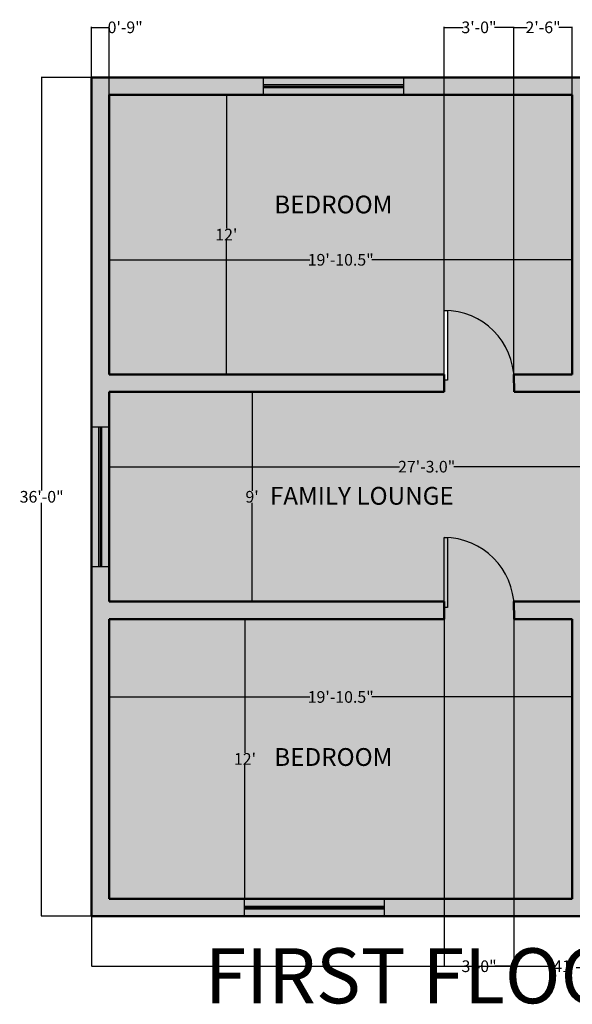
# Model space of a CAD drawing. Units: inches. Extents: x 1379 to 6665, y -118 to 1026.
# Tile 27 of 29: x 6130 to 6415, y 26 to 533. Entities that reach past the tile are written whole.
import ezdxf

# ---------------------------------------------------------------- set-up
doc = ezdxf.new("R2010")
doc.units = ezdxf.units.IN
doc.header["$MEASUREMENT"] = 0
for name, color, linetype, lineweight in [('A-ANNO-DIMS', 2, 'Continuous', 18), ('A-ANNO-TEXT', 7, 'Continuous', 35), ('A-AREA-IDEN', 7, 'Continuous', 25), ('A-DOOR', 1, 'Continuous', 25), ('A-FLOR-PATT', 252, 'Continuous', 13), ('A-GLAZ', 2, 'Continuous', 25), ('A-WALL', 7, 'Continuous', 50), ('A-WALL-PATT', 8, 'Continuous', 13)]:
    doc.layers.add(name, color=color, linetype=linetype, lineweight=lineweight)
doc.styles.get("Standard").update_dxf_attribs({"font": 'arial.ttf'})
doc.dimstyles.get("Standard").update_dxf_attribs({"dimtxt": 6, "dimasz": 0.18, "dimexe": 0.18, "dimexo": 0.0625, "dimgap": 0.09, "dimtad": 0, "dimtih": 1, "dimtoh": 1, "dimdec": 1, "dimzin": 0, "dimdsep": 46, "dimlunit": 3, "dimtxsty": 'Standard', "dimcen": 0.09, "dimclrt": 250, "dimadec": 0, "dimazin": 0, "dimtfac": 1, "dimtdec": 1, "dimtofl": 0, "dimtmove": 0, "dimatfit": 3, "dimfxl": 1, "dimtolj": 1, "dimtzin": 0, "dimarcsym": 0})

# ---------------------------------------------------------------- blocks, each defined once
blk = doc.blocks.new('*U3')
for p, q in [((0, 0), (0, -6)), ((36, 0), (36, -6))]:
    blk.add_line(p, q)
blk.add_lwpolyline([(0, 0), (0, 36), (1.75, 36), (1.75, 0)], close=True)
blk.add_arc((0, 0), 36, 0, 90)
blk = doc.blocks.new('*D76')
at = {"layer": 'A-ANNO-DIMS', "color": 0, "lineweight": -2, "transparency": 16777216}
for p, q in [((6235.37, 494.64), (6236.93, 494.64)), ((6236.75, 494.46), (6236.75, 425.74)), ((6236.75, 350.82), (6236.75, 419.54)), ((6235.37, 350.64), (6236.93, 350.64))]:
    blk.add_line(p, q, dxfattribs=at)
at = {"layer": 'A-ANNO-DIMS', "color": 0, "transparency": 16777216}
for points in [[(6236.72, 494.46), (6236.78, 494.46), (6236.75, 494.64)], [(6236.72, 350.82), (6236.78, 350.82), (6236.75, 350.64)]]:
    blk.add_solid(points, dxfattribs=at)
at = {"layer": 'Defpoints', "color": 0, "transparency": 16777216}
for p in [(6235.31, 494.64), (6235.31, 350.64), (6236.75, 350.64)]:
    blk.add_point(p, dxfattribs=at)
at = {"layer": 'A-ANNO-DIMS', "color": 0, "transparency": 16777216, "insert": (6236.75, 422.64), "char_height": 6, "attachment_point": 5}
blk.add_mtext("\\A1;12'", dxfattribs=at)
blk = doc.blocks.new('*D77')
at = {"layer": 'A-ANNO-DIMS', "color": 0, "lineweight": -2, "transparency": 16777216}
for p, q in [((6176.4, 417.36), (6176.4, 409.5)), ((6414.9, 417.36), (6414.9, 409.5)), ((6176.58, 409.68), (6279.71, 409.68)), ((6414.72, 409.68), (6311.59, 409.68))]:
    blk.add_line(p, q, dxfattribs=at)
at = {"layer": 'A-ANNO-DIMS', "color": 0, "transparency": 16777216}
for points in [[(6176.58, 409.71), (6176.58, 409.65), (6176.4, 409.68)], [(6414.72, 409.71), (6414.72, 409.65), (6414.9, 409.68)]]:
    blk.add_solid(points, dxfattribs=at)
at = {"layer": 'Defpoints', "color": 0, "transparency": 16777216}
for p in [(6176.4, 417.42), (6414.9, 417.42), (6414.9, 409.68)]:
    blk.add_point(p, dxfattribs=at)
at = {"layer": 'A-ANNO-DIMS', "color": 0, "transparency": 16777216, "insert": (6295.65, 409.68), "char_height": 6, "attachment_point": 5}
blk.add_mtext('\\A1;19\'-10.5"', dxfattribs=at)
blk = doc.blocks.new('*D78')
at = {"layer": 'A-ANNO-DIMS', "color": 0, "lineweight": -2, "transparency": 16777216}
for p, q in [((6281.87, 341.64), (6249.82, 341.64)), ((6250, 341.46), (6250, 290.79)), ((6250, 233.82), (6250, 284.49)), ((6281.87, 233.64), (6249.82, 233.64))]:
    blk.add_line(p, q, dxfattribs=at)
at = {"layer": 'A-ANNO-DIMS', "color": 0, "transparency": 16777216}
for points in [[(6249.97, 341.46), (6250.03, 341.46), (6250, 341.64)], [(6249.97, 233.82), (6250.03, 233.82), (6250, 233.64)]]:
    blk.add_solid(points, dxfattribs=at)
at = {"layer": 'Defpoints', "color": 0, "transparency": 16777216}
for p in [(6281.94, 341.64), (6250, 233.64), (6281.94, 233.64)]:
    blk.add_point(p, dxfattribs=at)
at = {"layer": 'A-ANNO-DIMS', "color": 0, "transparency": 16777216, "insert": (6250, 287.64), "char_height": 6, "attachment_point": 5}
blk.add_mtext("\\A1;9'", dxfattribs=at)
blk = doc.blocks.new('*D80')
at = {"layer": 'A-ANNO-DIMS', "color": 0, "lineweight": -2, "transparency": 16777216}
for p, q in [((6176.4, 282.22), (6176.4, 303.33)), ((6176.58, 303.15), (6325.96, 303.15)), ((6503.22, 303.15), (6353.84, 303.15)), ((6503.4, 282.22), (6503.4, 303.33))]:
    blk.add_line(p, q, dxfattribs=at)
at = {"layer": 'A-ANNO-DIMS', "color": 0, "transparency": 16777216}
for points in [[(6176.58, 303.18), (6176.58, 303.12), (6176.4, 303.15)], [(6503.22, 303.18), (6503.22, 303.12), (6503.4, 303.15)]]:
    blk.add_solid(points, dxfattribs=at)
at = {"layer": 'Defpoints', "color": 0, "transparency": 16777216}
for p in [(6503.4, 303.15), (6176.4, 282.16), (6503.4, 282.16)]:
    blk.add_point(p, dxfattribs=at)
at = {"layer": 'A-ANNO-DIMS', "color": 0, "transparency": 16777216, "insert": (6339.9, 303.15), "char_height": 6, "attachment_point": 5}
blk.add_mtext('\\A1;27\'-3.0"', dxfattribs=at)
blk = doc.blocks.new('*D87')
at = {"layer": 'A-ANNO-DIMS', "color": 0, "lineweight": -2, "transparency": 16777216}
for p, q in [((6262.59, 224.64), (6246.17, 224.64)), ((6246.35, 224.46), (6246.35, 155.74)), ((6246.35, 80.82), (6246.35, 149.54)), ((6262.59, 80.64), (6246.17, 80.64))]:
    blk.add_line(p, q, dxfattribs=at)
at = {"layer": 'A-ANNO-DIMS', "color": 0, "transparency": 16777216}
for points in [[(6246.32, 224.46), (6246.38, 224.46), (6246.35, 224.64)], [(6246.32, 80.82), (6246.38, 80.82), (6246.35, 80.64)]]:
    blk.add_solid(points, dxfattribs=at)
at = {"layer": 'Defpoints', "color": 0, "transparency": 16777216}
for p in [(6262.65, 224.64), (6246.35, 80.64), (6262.65, 80.64)]:
    blk.add_point(p, dxfattribs=at)
at = {"layer": 'A-ANNO-DIMS', "color": 0, "transparency": 16777216, "insert": (6246.35, 152.64), "char_height": 6, "attachment_point": 5}
blk.add_mtext("\\A1;12'", dxfattribs=at)
blk = doc.blocks.new('*D88')
at = {"layer": 'A-ANNO-DIMS', "color": 0, "lineweight": -2, "transparency": 16777216}
for p, q in [((6176.4, 163.43), (6176.4, 184.73)), ((6176.58, 184.55), (6279.71, 184.55)), ((6414.72, 184.55), (6311.59, 184.55)), ((6414.9, 164.7), (6414.9, 184.73))]:
    blk.add_line(p, q, dxfattribs=at)
at = {"layer": 'A-ANNO-DIMS', "color": 0, "transparency": 16777216}
for points in [[(6176.58, 184.58), (6176.58, 184.52), (6176.4, 184.55)], [(6414.72, 184.58), (6414.72, 184.52), (6414.9, 184.55)]]:
    blk.add_solid(points, dxfattribs=at)
at = {"layer": 'Defpoints', "color": 0, "transparency": 16777216}
for p in [(6414.9, 184.55), (6176.4, 163.37), (6414.9, 164.64)]:
    blk.add_point(p, dxfattribs=at)
at = {"layer": 'A-ANNO-DIMS', "color": 0, "transparency": 16777216, "insert": (6295.65, 184.55), "char_height": 6, "attachment_point": 5}
blk.add_mtext('\\A1;19\'-10.5"', dxfattribs=at)
blk = doc.blocks.new('WIN-1800')
for p, q in [((0, 0.73), (72, 0.73)), ((0, 0), (72, 0))]:
    blk.add_line(p, q)
blk = doc.blocks.new('*D136')
at = {"layer": 'A-ANNO-DIMS', "color": 0, "lineweight": -2, "transparency": 16777216}
for p, q in [((6167.4, 71.58), (6167.4, 45.71)), ((6665.4, 71.58), (6665.4, 45.71)), ((6167.58, 45.89), (6405.89, 45.89)), ((6665.22, 45.89), (6426.92, 45.89))]:
    blk.add_line(p, q, dxfattribs=at)
at = {"layer": 'A-ANNO-DIMS', "color": 0, "transparency": 16777216}
for points in [[(6167.58, 45.92), (6167.58, 45.86), (6167.4, 45.89)], [(6665.22, 45.92), (6665.22, 45.86), (6665.4, 45.89)]]:
    blk.add_solid(points, dxfattribs=at)
at = {"layer": 'Defpoints', "color": 0, "transparency": 16777216}
for p in [(6167.4, 71.64), (6665.4, 71.64), (6665.4, 45.89)]:
    blk.add_point(p, dxfattribs=at)
at = {"layer": 'A-ANNO-DIMS', "color": 250, "transparency": 16777216, "insert": (6416.4, 45.89), "char_height": 6, "attachment_point": 5}
blk.add_mtext('\\A1;41\'-6"', dxfattribs=at)
blk = doc.blocks.new('*D137')
at = {"layer": 'A-ANNO-DIMS', "color": 0, "lineweight": -2, "transparency": 16777216}
for p, q in [((6167.34, 503.64), (6141.47, 503.64)), ((6141.65, 503.46), (6141.65, 290.8)), ((6141.65, 71.82), (6141.65, 284.48)), ((6167.34, 71.64), (6141.47, 71.64))]:
    blk.add_line(p, q, dxfattribs=at)
at = {"layer": 'A-ANNO-DIMS', "color": 0, "transparency": 16777216}
for points in [[(6141.62, 503.46), (6141.68, 503.46), (6141.65, 503.64)], [(6141.62, 71.82), (6141.68, 71.82), (6141.65, 71.64)]]:
    blk.add_solid(points, dxfattribs=at)
at = {"layer": 'Defpoints', "color": 0, "transparency": 16777216}
for p in [(6141.65, 503.64), (6167.4, 503.64), (6167.4, 71.64)]:
    blk.add_point(p, dxfattribs=at)
at = {"layer": 'A-ANNO-DIMS', "color": 250, "transparency": 16777216, "insert": (6141.65, 287.64), "char_height": 6, "attachment_point": 5}
blk.add_mtext('\\A1;36\'-0"', dxfattribs=at)
blk = doc.blocks.new('*D138')
at = {"layer": 'A-ANNO-DIMS', "color": 0, "lineweight": -2, "transparency": 16777216}
for p, q in [((6167.4, 503.7), (6167.4, 529.57)), ((6167.58, 529.39), (6176.22, 529.39)), ((6176.4, 494.7), (6176.4, 529.57)), ((6176.4, 529.39), (6176.58, 529.39))]:
    blk.add_line(p, q, dxfattribs=at)
at = {"layer": 'A-ANNO-DIMS', "color": 0, "transparency": 16777216}
for points in [[(6167.58, 529.42), (6167.58, 529.36), (6167.4, 529.39)], [(6176.22, 529.42), (6176.22, 529.36), (6176.4, 529.39)]]:
    blk.add_solid(points, dxfattribs=at)
at = {"layer": 'Defpoints', "color": 0, "transparency": 16777216}
for p in [(6176.4, 529.39), (6167.4, 503.64), (6176.4, 494.64)]:
    blk.add_point(p, dxfattribs=at)
at = {"layer": 'A-ANNO-DIMS', "color": 250, "transparency": 16777216, "insert": (6184.65, 529.39), "char_height": 6, "attachment_point": 5}
blk.add_mtext('\\A1;0\'-9"', dxfattribs=at)
blk = doc.blocks.new('*D143')
at = {"layer": 'A-ANNO-DIMS', "color": 0, "lineweight": -2, "transparency": 16777216}
for p, q in [((6384.78, 350.7), (6384.78, 529.57)), ((6384.96, 529.39), (6391.72, 529.39)), ((6414.72, 529.39), (6407.96, 529.39)), ((6414.9, 350.7), (6414.9, 529.57))]:
    blk.add_line(p, q, dxfattribs=at)
at = {"layer": 'A-ANNO-DIMS', "color": 0, "transparency": 16777216}
for points in [[(6384.96, 529.42), (6384.96, 529.36), (6384.78, 529.39)], [(6414.72, 529.42), (6414.72, 529.36), (6414.9, 529.39)]]:
    blk.add_solid(points, dxfattribs=at)
at = {"layer": 'Defpoints', "color": 0, "transparency": 16777216}
for p in [(6414.9, 529.39), (6384.78, 350.64), (6414.9, 350.64)]:
    blk.add_point(p, dxfattribs=at)
at = {"layer": 'A-ANNO-DIMS', "color": 250, "transparency": 16777216, "insert": (6399.84, 529.39), "char_height": 6, "attachment_point": 5}
blk.add_mtext('\\A1;2\'-6"', dxfattribs=at)
blk = doc.blocks.new('*D144')
at = {"layer": 'A-ANNO-DIMS', "color": 0, "lineweight": -2, "transparency": 16777216}
for p, q in [((6348.9, 350.7), (6348.9, 529.57)), ((6349.08, 529.39), (6358.78, 529.39)), ((6384.6, 529.39), (6374.9, 529.39)), ((6384.78, 350.7), (6384.78, 529.57))]:
    blk.add_line(p, q, dxfattribs=at)
at = {"layer": 'A-ANNO-DIMS', "color": 0, "transparency": 16777216}
for points in [[(6349.08, 529.42), (6349.08, 529.36), (6348.9, 529.39)], [(6384.6, 529.42), (6384.6, 529.36), (6384.78, 529.39)]]:
    blk.add_solid(points, dxfattribs=at)
at = {"layer": 'Defpoints', "color": 0, "transparency": 16777216}
for p in [(6384.78, 529.39), (6348.9, 350.64), (6384.78, 350.64)]:
    blk.add_point(p, dxfattribs=at)
at = {"layer": 'A-ANNO-DIMS', "color": 250, "transparency": 16777216, "insert": (6366.84, 529.39), "char_height": 6, "attachment_point": 5}
blk.add_mtext('\\A1;3\'-0"', dxfattribs=at)
blk = doc.blocks.new('*D145')
at = {"layer": 'A-ANNO-DIMS', "color": 0, "lineweight": -2, "transparency": 16777216}
for p, q in [((6348.9, 233.58), (6348.9, 45.71)), ((6384.87, 233.58), (6384.87, 45.71)), ((6349.08, 45.89), (6358.82, 45.89)), ((6384.69, 45.89), (6374.95, 45.89))]:
    blk.add_line(p, q, dxfattribs=at)
at = {"layer": 'A-ANNO-DIMS', "color": 0, "transparency": 16777216}
for points in [[(6349.08, 45.92), (6349.08, 45.86), (6348.9, 45.89)], [(6384.69, 45.92), (6384.69, 45.86), (6384.87, 45.89)]]:
    blk.add_solid(points, dxfattribs=at)
at = {"layer": 'Defpoints', "color": 0, "transparency": 16777216}
for p in [(6348.9, 233.64), (6384.87, 233.64), (6384.87, 45.89)]:
    blk.add_point(p, dxfattribs=at)
at = {"layer": 'A-ANNO-DIMS', "color": 250, "transparency": 16777216, "insert": (6366.89, 45.89), "char_height": 6, "attachment_point": 5}
blk.add_mtext('\\A1;3\'-0"', dxfattribs=at)

msp = doc.modelspace()

# ---------------------------------------------------------------- hatches: boundary and pattern name
at = {"layer": 'A-FLOR-PATT', "transparency": 33554590}
h = msp.add_hatch(color=256, dxfattribs=at)
h.dxf.hatch_style = 1
h.paths.add_polyline_path([(6176.4, 382.14), (6176.4, 494.64), (6255.9, 494.64), (6255.9, 503.64), (6167.4, 503.64), (6167.4, 391.14), (6167.4, 323.64), (6176.4, 323.64), (6176.4, 341.64), (6348.9, 341.64), (6348.9, 350.64), (6176.4, 350.64)])
h.paths.add_polyline_path([(6348.9, 233.64), (6176.4, 233.64), (6176.4, 251.64), (6167.4, 251.64), (6167.4, 71.64), (6246.02, 71.64), (6246.02, 80.64), (6176.4, 80.64), (6176.4, 224.64), (6348.9, 224.64)])
h.paths.add_polyline_path([(6443.4, 80.64), (6419.4, 80.64), (6419.4, 164.64), (6467.4, 164.64), (6467.4, 169.14), (6419.4, 169.14), (6419.4, 224.64), (6419.4, 233.64), (6384.87, 233.64), (6384.9, 224.64), (6414.9, 224.64), (6414.9, 80.64), (6318.02, 80.64), (6318.02, 71.64), (6443.4, 71.64)])
h.paths.add_polyline_path([(6552.9, 80.64), (6500.4, 80.64), (6500.4, 169.14), (6491.4, 169.14), (6491.4, 164.64), (6491.4, 80.64), (6467.4, 80.64), (6467.4, 71.64), (6503.4, 71.64), (6552.9, 71.64)])
h.paths.add_polyline_path([(6665.4, 188.64), (6656.4, 188.64), (6656.4, 176.64), (6626.4, 176.64), (6626.4, 172.14), (6656.4, 172.14), (6656.4, 80.64), (6624.9, 80.64), (6624.9, 71.64), (6665.4, 71.64)])
h.paths.add_polyline_path([(6665.4, 503.64), (6614.4, 503.64), (6614.4, 494.64), (6656.4, 494.64), (6656.4, 374.64), (6608.4, 374.64), (6608.4, 370.14), (6656.4, 370.14), (6656.4, 331.14), (6512.4, 331.14), (6503.4, 331.14), (6503.4, 322.14), (6503.4, 317.64), (6656.4, 317.64), (6656.4, 233.64), (6503.4, 233.64), (6455.4, 233.64), (6455.4, 224.64), (6503.4, 224.64), (6567.9, 224.64), (6567.9, 176.64), (6540.4, 176.64), (6540.4, 172.14), (6567.9, 172.14), (6602.4, 172.14), (6602.4, 176.64), (6572.4, 176.64), (6572.4, 224.64), (6656.4, 224.64), (6656.4, 212.64), (6665.4, 212.64)])
h.paths.add_polyline_path([(6584.4, 374.64), (6536.4, 374.64), (6536.4, 370.14), (6536.4, 331.14), (6540.9, 331.14), (6540.9, 370.14), (6584.4, 370.14)], flags=17)
h.paths.add_polyline_path([(6500.4, 494.64), (6542.4, 494.64), (6542.4, 503.64), (6467.4, 503.64), (6467.4, 494.64), (6491.4, 494.64), (6491.4, 370.14), (6500.4, 370.14), (6500.4, 374.64)], flags=17)
h.paths.add_polyline_path([(6443.4, 503.64), (6407.4, 503.64), (6327.9, 503.64), (6327.9, 494.64), (6407.4, 494.64), (6414.9, 494.64), (6414.9, 350.64), (6384.78, 350.64), (6384.9, 341.64), (6419.4, 341.64), (6419.4, 406.14), (6467.4, 406.14), (6467.4, 410.64), (6419.4, 410.64), (6419.4, 494.64), (6443.4, 494.64)])
at = {"layer": 'A-WALL-PATT', "transparency": 33554564}
h = msp.add_hatch(color=256, dxfattribs=at)
h.dxf.hatch_style = 1
h.paths.add_polyline_path([(6327.9, 503.64), (6255.9, 503.64), (6255.9, 499.87), (6327.9, 499.87)])
h.paths.add_polyline_path([(6327.9, 499.14), (6255.9, 499.14), (6255.9, 498.41), (6327.9, 498.41)])
h.paths.add_polyline_path([(6327.9, 499.87), (6255.9, 499.87), (6255.9, 499.14), (6327.9, 499.14)])
h.paths.add_polyline_path([(6327.9, 498.41), (6255.9, 498.41), (6255.9, 494.64), (6327.9, 494.64)])
at = {"layer": 'A-WALL-PATT', "transparency": 33554590}
h = msp.add_hatch(color=256, dxfattribs=at)
h.dxf.hatch_style = 1
h.paths.add_polyline_path([(6414.9, 494.64), (6176.4, 494.64), (6176.4, 382.14), (6176.4, 350.64), (6348.9, 350.64), (6348.9, 383.64), (6350.65, 383.64), (6350.65, 383.6, -0.376042), (6384.78, 350.64), (6414.9, 350.64)])
h.paths.add_polyline_path([(6503.4, 317.64), (6503.4, 322.14), (6503.4, 331.14), (6512.4, 331.14), (6536.4, 331.14), (6536.4, 370.14), (6536.4, 376.14, 0.400041), (6502.15, 412.1), (6502.15, 376.14), (6500.4, 376.14), (6500.4, 370.14), (6491.4, 370.14), (6491.4, 414.39, 0.392996), (6469.15, 438.33), (6469.15, 414.39), (6467.4, 414.39), (6467.4, 408.39), (6467.4, 406.14), (6419.4, 406.14), (6419.4, 341.64), (6384.9, 341.64), (6384.78, 350.64, 0.376042), (6350.65, 383.6), (6350.65, 347.64), (6348.9, 347.64), (6348.9, 341.64), (6176.4, 341.64), (6176.4, 233.64), (6348.9, 233.64), (6348.9, 266.64), (6350.65, 266.64), (6350.65, 266.6, -0.376042), (6384.78, 233.64), (6419.4, 233.64), (6419.4, 224.64), (6419.4, 169.14), (6467.4, 169.14), (6467.4, 172.89), (6467.4, 196.89), (6469.15, 196.89), (6469.15, 196.83, -0.392996), (6491.4, 172.89), (6491.4, 169.14), (6500.4, 169.14), (6500.4, 175.14), (6500.4, 215.14), (6502.15, 215.14), (6502.15, 215.1, -0.390605), (6540.37, 176.64), (6567.9, 176.64), (6567.9, 224.64), (6500.4, 224.64), (6455.4, 224.64), (6455.4, 233.64), (6503.4, 233.64), (6503.4, 275.64)])
h.paths.add_polyline_path([(6491.4, 494.64), (6419.4, 494.64), (6419.4, 410.64), (6467.4, 410.64), (6467.4, 414.39), (6467.4, 438.39), (6469.15, 438.39), (6469.15, 438.33, -0.392996), (6491.4, 414.39)])
h.paths.add_polyline_path([(6656.4, 494.64), (6500.4, 494.64), (6500.4, 412.14), (6502.15, 412.14), (6502.15, 412.1, -0.400041), (6536.4, 376.14), (6536.4, 374.64), (6584.4, 374.64), (6584.4, 376.14), (6584.4, 400.14), (6586.15, 400.14), (6586.15, 400.08, -0.392996), (6608.4, 376.14), (6608.4, 374.64), (6656.4, 374.64)])
h.paths.add_polyline_path([(6414.9, 224.64), (6384.9, 224.64), (6384.87, 233.64), (6384.78, 233.64, 0.376042), (6350.65, 266.6), (6350.65, 266.64), (6348.9, 266.64), (6348.9, 233.64), (6348.9, 224.64), (6176.4, 224.64), (6176.4, 80.64), (6414.9, 80.64)])
h.paths.add_polyline_path([(6491.4, 164.64), (6491.4, 169.14), (6491.4, 172.89, 0.392996), (6469.15, 196.83), (6469.15, 172.89), (6467.4, 172.89), (6467.4, 169.14), (6467.4, 166.89), (6467.4, 164.64), (6419.4, 164.64), (6419.4, 80.64), (6491.4, 80.64)])
h.paths.add_polyline_path([(6656.4, 172.14), (6626.4, 172.14), (6626.4, 178.14, 0.392996), (6604.15, 202.08), (6604.15, 178.14), (6602.4, 178.14), (6602.4, 172.14), (6567.9, 172.14), (6540.4, 172.14), (6540.4, 175.14, 0.401453), (6502.15, 215.1), (6502.15, 175.14), (6500.4, 175.14), (6500.4, 169.14), (6500.4, 80.64), (6503.4, 80.64), (6656.4, 80.64)])
h.paths.add_polyline_path([(6656.4, 224.64), (6572.4, 224.64), (6572.4, 176.64), (6602.4, 176.64), (6602.4, 178.14), (6602.4, 202.14), (6604.15, 202.14), (6604.15, 202.08, -0.392996), (6626.4, 178.14), (6626.4, 176.64), (6656.4, 176.64)])
h.paths.add_polyline_path([(6656.4, 370.14), (6608.4, 370.14), (6608.4, 376.14, 0.392996), (6586.15, 400.08), (6586.15, 376.14), (6584.4, 376.14), (6584.4, 374.64), (6584.4, 370.14), (6540.9, 370.14), (6540.9, 331.14), (6656.4, 331.14)])
h.paths.add_polyline_path([(6259.03, 431.04), (6329.97, 431.04), (6329.97, 445.28), (6259.03, 445.28)], flags=24)
h.paths.add_polyline_path([(6256.77, 281.02), (6365.45, 281.02), (6365.45, 295.25), (6256.77, 295.25)], flags=24)
h.paths.add_polyline_path([(6437.04, 454.45), (6486.63, 454.45), (6486.63, 468.69), (6437.04, 468.69)], flags=24)
h.paths.add_polyline_path([(6549.24, 450.74), (6620.18, 450.74), (6620.18, 464.98), (6549.24, 464.98)], flags=24)
h.paths.add_polyline_path([(6259.03, 146.52), (6329.97, 146.52), (6329.97, 160.75), (6259.03, 160.75)], flags=24)
h.paths.add_polyline_path([(6431.31, 122.15), (6480.89, 122.15), (6480.89, 136.39), (6431.31, 136.39)], flags=24)
h.paths.add_polyline_path([(6550.53, 122.44), (6621.47, 122.44), (6621.47, 136.68), (6550.53, 136.68)], flags=24)
h.paths.add_polyline_path([(6590.78, 206.76), (6640.36, 206.76), (6640.36, 221), (6590.78, 221)], flags=24)
h.paths.add_polyline_path([(6574.95, 341.57), (6624.53, 341.57), (6624.53, 355.8), (6574.95, 355.8)], flags=24)
at = {"layer": 'A-WALL-PATT', "transparency": 33554564}
h = msp.add_hatch(color=256, dxfattribs=at)
h.dxf.hatch_style = 1
h.paths.add_polyline_path([(6167.4, 323.64), (6167.4, 251.64), (6171.17, 251.64), (6171.17, 323.64)])
h.paths.add_polyline_path([(6171.9, 323.64), (6171.9, 251.64), (6172.63, 251.64), (6172.63, 323.64)])
h.paths.add_polyline_path([(6171.17, 323.64), (6171.17, 251.64), (6171.9, 251.64), (6171.9, 323.64)])
h.paths.add_polyline_path([(6172.63, 323.64), (6172.63, 251.64), (6176.4, 251.64), (6176.4, 323.64)])
h = msp.add_hatch(color=256, dxfattribs=at)
h.dxf.hatch_style = 1
h.paths.add_polyline_path([(6318.02, 80.64), (6246.02, 80.64), (6246.02, 76.87), (6318.02, 76.87)])
h.paths.add_polyline_path([(6318.02, 76.14), (6246.02, 76.14), (6246.02, 75.41), (6318.02, 75.41)])
h.paths.add_polyline_path([(6318.02, 76.87), (6246.02, 76.87), (6246.02, 76.14), (6318.02, 76.14)])
h.paths.add_polyline_path([(6318.02, 75.41), (6246.02, 75.41), (6246.02, 71.64), (6318.02, 71.64)])

# ---------------------------------------------------------------- linework, layer by layer
at = {"layer": 'A-GLAZ'}
for p, q in [((6255.9, 498.41), (6327.9, 498.41)), ((6172.63, 251.64), (6172.63, 323.64)), ((6246.02, 75.41), (6318.02, 75.41))]:
    msp.add_line(p, q, dxfattribs=at)
for points in [[(6255.9, 503.64), (6327.9, 503.64), (6327.9, 494.64), (6255.9, 494.64)], [(6167.4, 251.64), (6167.4, 323.64), (6176.4, 323.64), (6176.4, 251.64)], [(6246.02, 80.64), (6318.02, 80.64), (6318.02, 71.64), (6246.02, 71.64)]]:
    msp.add_lwpolyline(points, close=True, dxfattribs=at)
at = {"layer": 'A-WALL'}
for p, q in [((6167.4, 391.14), (6167.4, 503.64)), ((6167.4, 503.64), (6407.4, 503.64)), ((6665.4, 503.64), (6407.4, 503.64)), ((6414.9, 494.64), (6176.4, 494.64)), ((6176.4, 382.14), (6176.4, 494.64)), ((6176.4, 494.64), (6407.4, 494.64)), ((6414.9, 350.64), (6414.9, 494.64)), ((6167.4, 391.14), (6167.4, 71.64)), ((6176.4, 382.14), (6176.4, 350.64)), ((6348.9, 350.64), (6176.4, 350.64)), ((6348.9, 341.64), (6348.9, 350.64)), ((6414.9, 350.64), (6384.78, 350.64)), ((6384.9, 341.64), (6384.78, 350.64)), ((6176.4, 341.64), (6176.4, 233.64)), ((6348.9, 341.64), (6176.4, 341.64)), ((6419.4, 341.64), (6384.9, 341.64)), ((6348.9, 233.64), (6176.4, 233.64)), ((6348.9, 224.64), (6348.9, 233.64)), ((6419.4, 233.64), (6384.87, 233.64)), ((6384.87, 233.64), (6384.9, 224.64)), ((6348.9, 224.64), (6176.4, 224.64)), ((6176.4, 224.64), (6176.4, 80.64)), ((6414.9, 224.64), (6384.9, 224.64)), ((6414.9, 224.64), (6414.9, 80.64)), ((6414.9, 80.64), (6176.4, 80.64)), ((6503.4, 71.64), (6167.4, 71.64))]:
    msp.add_line(p, q, dxfattribs=at)

# ---------------------------------------------------------------- block references
at = {"layer": 'A-DOOR'}
for p in [(6348.9, 347.64), (6348.9, 230.64)]:
    msp.add_blockref('*U3', p, dxfattribs=at)
at = {"layer": 'A-GLAZ'}
for p in [(6255.9, 499.14), (6246.02, 76.14)]:
    msp.add_blockref('WIN-1800', p, dxfattribs=at)
at = {"layer": 'A-GLAZ', "rotation": 89.99999999999936}
msp.add_blockref('WIN-1800', (6171.9, 251.64), dxfattribs=at)

# ---------------------------------------------------------------- texts
at = {"layer": 'A-ANNO-TEXT'}
msp.add_text('FIRST FLOOR PLAN', height=28.3655, dxfattribs=at).set_placement((6225.6, 26.79))
at = {"layer": 'A-AREA-IDEN'}
for s, height, p in [('BEDROOM', 9.17, (6261.4, 433.57)), ('FAMILY LOUNGE', 9.1702, (6259.15, 283.55)), ('BEDROOM', 9.17, (6261.4, 149.05))]:
    msp.add_text(s, height=height, dxfattribs=at).set_placement(p)

# ---------------------------------------------------------------- dimensions: what is measured, and where the dimension line sits
at = {"layer": 'A-ANNO-DIMS'}
for base, p1, p2, override, picture, middle in [((6176.4, 529.39), (6167.4, 503.64), (6176.4, 494.64), {"dimdec": 1, "dimlfac": 1, "dimrnd": 0, "dimzin": 1, "dimdsep": 46, "dimlunit": 4, "dimfrac": 2}, '*D138', (6184.65, 529.39)), ((6384.78, 529.39), (6348.9, 350.64), (6384.78, 350.64), {"dimdec": 1, "dimlfac": 1, "dimrnd": 0, "dimzin": 1, "dimdsep": 46, "dimlunit": 4, "dimfrac": 2}, '*D144', (6366.84, 529.39)), ((6414.9, 529.39), (6384.78, 350.64), (6414.9, 350.64), {"dimdec": 1, "dimlfac": 1, "dimrnd": 0, "dimzin": 1, "dimdsep": 46, "dimlunit": 4, "dimfrac": 2}, '*D143', (6399.84, 529.39)), ((6414.9, 409.68), (6176.4, 417.42), (6414.9, 417.42), {"dimclrd": 0, "dimclre": 0, "dimclrt": 0}, '*D77', (6295.65, 409.68)), ((6503.4, 303.15), (6176.4, 282.16), (6503.4, 282.16), {"dimclrd": 0, "dimclre": 0, "dimclrt": 0}, '*D80', (6339.9, 303.15)), ((6384.87, 45.89), (6348.9, 233.64), (6384.87, 233.64), {"dimdec": 1, "dimlfac": 1, "dimrnd": 0, "dimzin": 1, "dimdsep": 46, "dimlunit": 4, "dimfrac": 2}, '*D145', (6366.89, 45.89)), ((6414.9, 184.55), (6176.4, 163.37), (6414.9, 164.64), {"dimclrd": 0, "dimclre": 0, "dimclrt": 0}, '*D88', (6295.65, 184.55)), ((6665.4, 45.89), (6167.4, 71.64), (6665.4, 71.64), {"dimdec": 1, "dimlfac": 1, "dimrnd": 0, "dimzin": 1, "dimdsep": 46, "dimlunit": 4, "dimfrac": 2}, '*D136', (6416.4, 45.89))]:
    dim = msp.add_linear_dim(base=base, p1=p1, p2=p2, dimstyle='Standard', override=override, dxfattribs=at)
    dim.commit()
    dim.dimension.update_dxf_attribs({"geometry": picture, "text_midpoint": middle})
for base, p1, p2, override, picture, middle in [((6141.65, 503.64), (6167.4, 71.64), (6167.4, 503.64), {"dimdec": 1, "dimlfac": 1, "dimrnd": 0, "dimzin": 1, "dimdsep": 46, "dimlunit": 4, "dimfrac": 2}, '*D137', (6141.65, 287.64)), ((6236.75, 350.64), (6235.31, 494.64), (6235.31, 350.64), {"dimclrd": 0, "dimclre": 0, "dimclrt": 0}, '*D76', (6236.75, 422.64)), ((6250, 233.64), (6281.94, 341.64), (6281.94, 233.64), {"dimclrd": 0, "dimclre": 0, "dimclrt": 0}, '*D78', (6250, 287.64)), ((6246.35, 80.64), (6262.65, 224.64), (6262.65, 80.64), {"dimclrd": 0, "dimclre": 0, "dimclrt": 0}, '*D87', (6246.35, 152.64))]:
    dim = msp.add_linear_dim(base=base, p1=p1, p2=p2, angle=90, dimstyle='Standard', override=override, dxfattribs=at)
    dim.commit()
    dim.dimension.update_dxf_attribs({"geometry": picture, "text_midpoint": middle})

doc.saveas('drawing.dxf')
